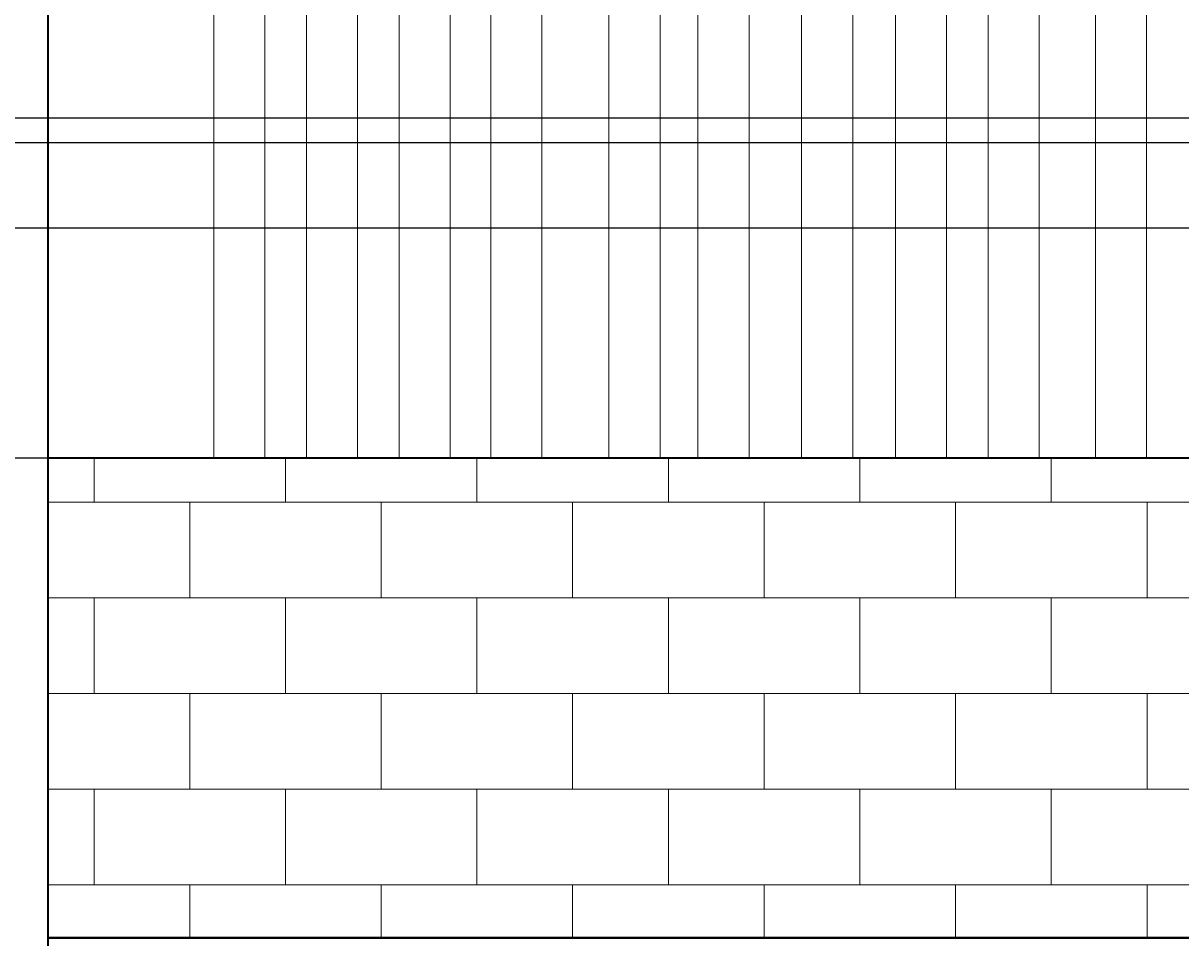
# Model space of a CAD drawing. Units: inches. Extents: x -13 to 809, y 112 to 656.
# Tile 22 of 55: x 339 to 430, y 251 to 323. Entities that reach past the tile are written whole.
import ezdxf

# ---------------------------------------------------------------- set-up
doc = ezdxf.new("R2010")
doc.units = ezdxf.units.IN
doc.header["$MEASUREMENT"] = 0
for name, color, linetype, lineweight in [('A-ANNO-DIMS', 2, 'Continuous', 18), ('A-ELEV', 7, 'Continuous', 35), ('A-ELEV-PATT', 8, 'Continuous', 13)]:
    doc.layers.add(name, color=color, linetype=linetype, lineweight=lineweight)
doc.styles.get("Standard").update_dxf_attribs({"font": 'arial.ttf'})
doc.dimstyles.get("Standard").update_dxf_attribs({"dimtxt": 0.625, "dimasz": 0.18, "dimexe": 0.18, "dimexo": 0.0625, "dimgap": 0.09, "dimtad": 0, "dimtih": 1, "dimtoh": 1, "dimdec": 4, "dimzin": 0, "dimdsep": 46, "dimlunit": 4, "dimtxsty": 'Standard', "dimcen": 0.09, "dimadec": 0, "dimazin": 0, "dimtfac": 1, "dimtdec": 4, "dimtofl": 0, "dimtmove": 0, "dimatfit": 3, "dimfxl": 1, "dimtolj": 1, "dimtzin": 0, "dimarcsym": 0})

# ---------------------------------------------------------------- blocks, each defined once
blk = doc.blocks.new('*D19')
at = {"layer": 'A-ANNO-DIMS', "color": 0, "lineweight": -2, "transparency": 16777216}
for p, q in [((337.507, 306.457), (337.507, 112.34)), ((365.938, 210.722), (365.938, 112.34)), ((337.687, 112.52), (350.573, 112.52)), ((365.758, 112.52), (352.873, 112.52))]:
    blk.add_line(p, q, dxfattribs=at)
at = {"layer": 'A-ANNO-DIMS', "color": 0, "transparency": 16777216}
for points in [[(337.687, 112.55), (337.687, 112.49), (337.507, 112.52)], [(365.758, 112.55), (365.758, 112.49), (365.938, 112.52)]]:
    blk.add_solid(points, dxfattribs=at)
at = {"layer": 'Defpoints', "color": 0, "transparency": 16777216}
for p in [(337.507, 306.52), (365.938, 210.785), (365.938, 112.52)]:
    blk.add_point(p, dxfattribs=at)
at = {"layer": 'A-ANNO-DIMS', "color": 0, "transparency": 16777216, "insert": (351.723, 112.52), "char_height": 0.625, "attachment_point": 5}
blk.add_mtext('\\A1;28.43', dxfattribs=at)
blk = doc.blocks.new('*D39')
at = {"layer": 'A-ANNO-DIMS', "color": 0, "lineweight": -2, "transparency": 16777216}
for p, q in [((341.345, 524.281), (-12.099, 524.281)), ((-11.919, 524.101), (-11.919, 406.775)), ((-11.919, 288.631), (-11.919, 405.957)), ((341.345, 288.451), (-12.099, 288.451))]:
    blk.add_line(p, q, dxfattribs=at)
at = {"layer": 'A-ANNO-DIMS', "color": 0, "transparency": 16777216}
for points in [[(-11.949, 524.101), (-11.889, 524.101), (-11.919, 524.281)], [(-11.949, 288.631), (-11.889, 288.631), (-11.919, 288.451)]]:
    blk.add_solid(points, dxfattribs=at)
at = {"layer": 'Defpoints', "color": 0, "transparency": 16777216}
for p in [(-11.919, 524.281), (341.407, 524.281), (341.407, 288.451)]:
    blk.add_point(p, dxfattribs=at)
at = {"layer": 'A-ANNO-DIMS', "color": 0, "transparency": 16777216, "insert": (-11.919, 406.366), "char_height": 0.625, "attachment_point": 5}
blk.add_mtext('\\A1;235.83', dxfattribs=at)
blk = doc.blocks.new('*D40')
at = {"layer": 'A-ANNO-DIMS', "color": 0, "lineweight": -2, "transparency": 16777216}
for p, q in [((471.037, 313.167), (-12.099, 313.167)), ((-11.919, 312.987), (-11.919, 301.218)), ((-11.919, 288.631), (-11.919, 300.4)), ((341.345, 288.451), (-12.099, 288.451))]:
    blk.add_line(p, q, dxfattribs=at)
at = {"layer": 'A-ANNO-DIMS', "color": 0, "transparency": 16777216}
for points in [[(-11.949, 312.987), (-11.889, 312.987), (-11.919, 313.167)], [(-11.949, 288.631), (-11.889, 288.631), (-11.919, 288.451)]]:
    blk.add_solid(points, dxfattribs=at)
at = {"layer": 'Defpoints', "color": 0, "transparency": 16777216}
for p in [(471.1, 313.167), (-11.919, 288.451), (341.407, 288.451)]:
    blk.add_point(p, dxfattribs=at)
at = {"layer": 'A-ANNO-DIMS', "color": 0, "transparency": 16777216, "insert": (-11.919, 300.809), "char_height": 0.625, "attachment_point": 5}
blk.add_mtext('\\A1;24.716', dxfattribs=at)
blk = doc.blocks.new('*D41')
at = {"layer": 'A-ANNO-DIMS', "color": 0, "lineweight": -2, "transparency": 16777216}
for p, q in [((471.037, 357.98), (-12.099, 357.98)), ((-11.919, 357.8), (-11.919, 335.983)), ((-11.919, 313.347), (-11.919, 335.164)), ((471.037, 313.167), (-12.099, 313.167))]:
    blk.add_line(p, q, dxfattribs=at)
at = {"layer": 'A-ANNO-DIMS', "color": 0, "transparency": 16777216}
for points in [[(-11.949, 357.8), (-11.889, 357.8), (-11.919, 357.98)], [(-11.949, 313.347), (-11.889, 313.347), (-11.919, 313.167)]]:
    blk.add_solid(points, dxfattribs=at)
at = {"layer": 'Defpoints', "color": 0, "transparency": 16777216}
for p in [(-11.919, 357.98), (471.1, 357.98), (471.1, 313.167)]:
    blk.add_point(p, dxfattribs=at)
at = {"layer": 'A-ANNO-DIMS', "color": 0, "transparency": 16777216, "insert": (-11.919, 335.574), "char_height": 0.625, "attachment_point": 5}
blk.add_mtext('\\A1;44.81', dxfattribs=at)
blk = doc.blocks.new('*D51')
at = {"layer": 'A-ANNO-DIMS', "color": 0, "lineweight": -2, "transparency": 16777216}
for p, q in [((341.407, 288.388), (341.407, 112.34)), ((442.184, 288.388), (442.184, 112.34)), ((341.587, 112.52), (390.437, 112.52)), ((442.004, 112.52), (393.154, 112.52))]:
    blk.add_line(p, q, dxfattribs=at)
at = {"layer": 'A-ANNO-DIMS', "color": 0, "transparency": 16777216}
for points in [[(341.587, 112.55), (341.587, 112.49), (341.407, 112.52)], [(442.004, 112.55), (442.004, 112.49), (442.184, 112.52)]]:
    blk.add_solid(points, dxfattribs=at)
at = {"layer": 'Defpoints', "color": 0, "transparency": 16777216}
for p in [(341.407, 288.451), (442.184, 288.451), (442.184, 112.52)]:
    blk.add_point(p, dxfattribs=at)
at = {"layer": 'A-ANNO-DIMS', "color": 0, "transparency": 16777216, "insert": (391.796, 112.52), "char_height": 0.625, "attachment_point": 5}
blk.add_mtext('\\A1;100.78', dxfattribs=at)
blk = doc.blocks.new('*D106')
at = {"layer": 'A-ANNO-DIMS', "color": 0, "lineweight": -2, "transparency": 16777216}
for p, q in [((319.57, 315.144), (807.769, 315.144)), ((807.589, 314.964), (807.589, 311.241)), ((807.589, 306.7), (807.589, 310.423)), ((337.57, 306.52), (807.769, 306.52))]:
    blk.add_line(p, q, dxfattribs=at)
at = {"layer": 'A-ANNO-DIMS', "color": 0, "transparency": 16777216}
for points in [[(807.559, 314.964), (807.619, 314.964), (807.589, 315.144)], [(807.559, 306.7), (807.619, 306.7), (807.589, 306.52)]]:
    blk.add_solid(points, dxfattribs=at)
at = {"layer": 'Defpoints', "color": 0, "transparency": 16777216}
for p in [(319.507, 315.144), (807.589, 315.144), (337.507, 306.52)]:
    blk.add_point(p, dxfattribs=at)
at = {"layer": 'A-ANNO-DIMS', "color": 0, "transparency": 16777216, "insert": (807.589, 310.832), "char_height": 0.625, "attachment_point": 5}
blk.add_mtext('\\A1;8.624', dxfattribs=at)

msp = doc.modelspace()

# ---------------------------------------------------------------- hatches: boundary and pattern name
at = {"layer": 'A-ELEV-PATT'}
h = msp.add_hatch(dxfattribs=at)
h.set_pattern_fill('BRICK', color=256, scale=30)
h.paths.add_polyline_path([(591.008, 558.5199), (341.4072, 558.5199), (341.4072, 524.281), (542.9617, 524.281), (542.9617, 288.4508), (341.4072, 288.4508), (341.4072, 250.8429), (591.008, 250.8429)])

# ---------------------------------------------------------------- linework, layer by layer
at = {"layer": 'A-ELEV'}
for p, q in [((341.4072, 210.7849), (341.4072, 524.281)), ((341.4072, 250.8429), (591.008, 250.8429))]:
    msp.add_line(p, q, dxfattribs=at)
for points in [[(341.4072, 558.5199), (591.008, 558.5199), (591.008, 250.8429), (341.4072, 250.8429)], [(341.4072, 524.281), (542.9617, 524.281), (542.9617, 288.4508), (341.4072, 288.4508)]]:
    msp.add_lwpolyline(points, close=True, dxfattribs=at)
at = {"layer": 'A-ELEV-PATT'}
for points in [[(354.3886, 288.4508), (354.3886, 523.3908), (354.3886, 524.281)], [(358.3886, 288.4508), (358.3886, 523.3908), (358.3886, 524.281)], [(361.6625, 288.4508), (361.6625, 523.3908), (361.6625, 524.281)], [(365.6625, 288.4508), (365.6625, 523.3908), (365.6625, 524.281)], [(368.9215, 288.4508), (368.9215, 523.3908), (368.9215, 524.281)], [(372.9215, 288.4508), (372.9215, 523.3908), (372.9215, 524.281)], [(376.0866, 288.4508), (376.0866, 523.3908), (376.0866, 524.281)], [(380.0866, 288.4508), (380.0866, 523.3908), (380.0866, 524.281)], [(385.3536, 288.4508), (385.3536, 523.3908), (385.3536, 524.281)], [(389.3536, 288.4508), (389.3536, 523.3908), (389.3536, 524.281)], [(392.3277, 288.4508), (392.3277, 523.3908), (392.3277, 524.281)], [(396.3277, 288.4508), (396.3277, 523.3908), (396.3277, 524.281)], [(400.4483, 288.4508), (400.4483, 523.3908), (400.4483, 524.281)], [(404.4483, 288.4508), (404.4483, 523.3908), (404.4483, 524.281)], [(407.8046, 288.4508), (407.8046, 523.3908), (407.8046, 524.281)], [(411.8046, 288.4508), (411.8046, 523.3908), (411.8046, 524.281)], [(415.0653, 288.4508), (415.0653, 523.3908), (415.0653, 524.281)], [(419.0653, 288.4508), (419.0653, 523.3908), (419.0653, 524.281)], [(423.4725, 288.4508), (423.4725, 523.3908), (423.4725, 524.281)], [(427.4725, 288.4508), (427.4725, 523.3908), (427.4725, 524.281)]]:
    msp.add_lwpolyline(points, dxfattribs=at)

# ---------------------------------------------------------------- dimensions: what is measured, and where the dimension line sits
at = {"layer": 'A-ANNO-DIMS'}
for base, p1, p2, override, picture, middle in [((-11.9191, 524.281), (341.4072, 288.4508), (341.4072, 524.281), {"dimdec": 2, "dimlfac": 1, "dimrnd": 0, "dimzin": 0, "dimdsep": 46, "dimlunit": 2}, '*D39', (-11.9191, 406.3659)), ((-11.9191, 357.9804), (471.0998, 313.1667), (471.0998, 357.9804), {"dimdec": 2, "dimlfac": 1, "dimrnd": 0, "dimzin": 0, "dimdsep": 46, "dimlunit": 2}, '*D41', (-11.9191, 335.5735)), ((807.5888, 315.1435), (337.5074, 306.5199), (319.5074, 315.1435), {"dimdec": 3, "dimlfac": 1, "dimrnd": 0, "dimzin": 0, "dimdsep": 46, "dimlunit": 2}, '*D106', (807.5888, 310.8317)), ((-11.9191, 288.4508), (471.0998, 313.1667), (341.4072, 288.4508), {"dimdec": 3, "dimlfac": 1, "dimrnd": 0, "dimzin": 0, "dimdsep": 46, "dimlunit": 2}, '*D40', (-11.9191, 300.8087))]:
    dim = msp.add_linear_dim(base=base, p1=p1, p2=p2, angle=90, dimstyle='Standard', override=override, dxfattribs=at)
    dim.commit()
    dim.dimension.update_dxf_attribs({"geometry": picture, "text_midpoint": middle})
for base, p1, p2, picture, middle in [((365.9383, 112.5199), (337.5074, 306.5199), (365.9383, 210.7849), '*D19', (351.7228, 112.5199)), ((442.1845, 112.5199), (341.4072, 288.4508), (442.1845, 288.4508), '*D51', (391.7958, 112.5199))]:
    dim = msp.add_linear_dim(base=base, p1=p1, p2=p2, dimstyle='Standard', override={"dimdec": 2, "dimlfac": 1, "dimrnd": 0, "dimzin": 0, "dimdsep": 46, "dimlunit": 2}, dxfattribs=at)
    dim.commit()
    dim.dimension.update_dxf_attribs({"geometry": picture, "text_midpoint": middle})

doc.saveas('drawing.dxf')
